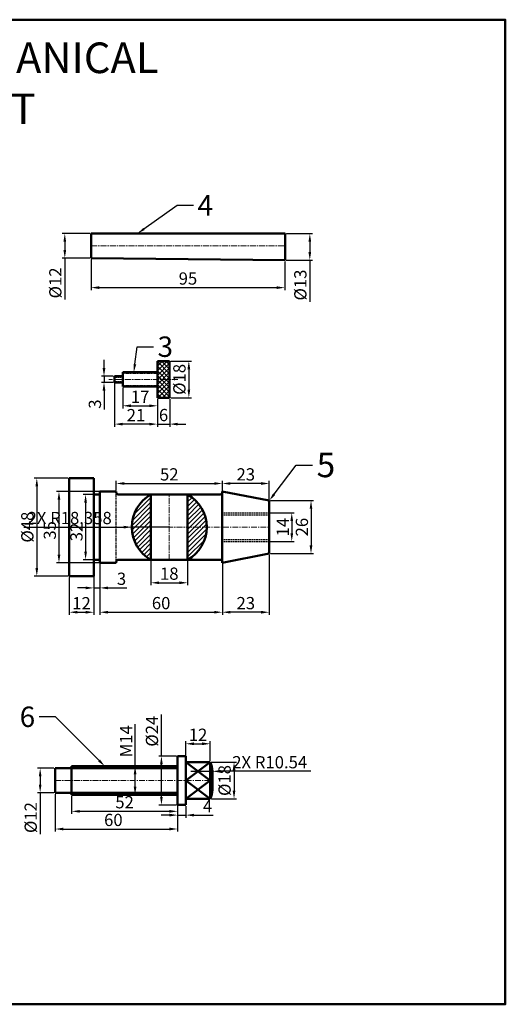
# Model space of a CAD drawing. Units: millimetres. Extents: x 197 to 841, y -182 to 351.
# Tile 3 of 3: x 603 to 841, y -132 to 351. Entities that reach past the tile are written whole.
import ezdxf
from ezdxf import colors
from ezdxf.entities.mleader import LeaderData, LeaderLine
from ezdxf.math import Vec2, Vec3

# ---------------------------------------------------------------- set-up
doc = ezdxf.new("R2010")
doc.units = ezdxf.units.MM
doc.header["$LTSCALE"] = 0.3
doc.linetypes.add('CENTER', pattern=[50.8, 31.75, -6.35, 6.35, -6.35])
doc.linetypes.add('HIDDEN', pattern=[9.525, 6.35, -3.175])
for name, color, linetype, lineweight in [('M-CNTR', 1, 'CENTER', 18), ('M-DIMS', 2, 'Continuous', 25), ('M-HATC', 8, 'Continuous', 18), ('M-HIDN', 6, 'HIDDEN', 25), ('M-OUTL', 7, 'Continuous', 50), ('M-TEXT', 3, 'Continuous', 25), ('M-TTLB', 7, 'Continuous', 50)]:
    doc.layers.add(name, color=color, linetype=linetype, lineweight=lineweight)
doc.styles.get("Standard").update_dxf_attribs({"font": 'arial.ttf'})
doc.dimstyles.new('ISO-25', dxfattribs={"dimtxt": 6, "dimasz": 4, "dimexe": 1.25, "dimexo": 0.625, "dimtad": 1, "dimdec": 0, "dimtxsty": 'Standard', "dimcen": 2.5, "dimadec": 0, "dimazin": 0, "dimtfac": 1, "dimtdec": 0, "dimtmove": 0, "dimatfit": 3, "dimfxl": 1, "dimarcsym": 0})

# ---------------------------------------------------------------- blocks, each defined once
blk = doc.blocks.new('*D37')
at = {"layer": 'Defpoints', "color": 0, "ltscale": 0.3, "transparency": 16777216}
for p in [(733.03, 245.93), (732.9, 232.93), (745.12, 232.93)]:
    blk.add_point(p, dxfattribs=at)
at = {"layer": 'M-DIMS', "color": 0, "lineweight": -2, "ltscale": 0.3, "transparency": 16777216}
for p, q in [((733.66, 245.93), (746.37, 245.93)), ((745.12, 241.93), (745.12, 236.93)), ((733.52, 232.93), (746.37, 232.93)), ((745.12, 232.93), (745.12, 212.55))]:
    blk.add_line(p, q, dxfattribs=at)
at = {"layer": 'M-DIMS', "color": 0, "ltscale": 0.3, "transparency": 16777216}
for points in [[(744.45, 241.93), (745.79, 241.93), (745.12, 245.93)], [(744.45, 236.93), (745.79, 236.93), (745.12, 232.93)]]:
    blk.add_solid(points, dxfattribs=at)
at = {"layer": 'M-DIMS', "color": 0, "ltscale": 0.3, "transparency": 16777216, "insert": (741.26, 220.74), "char_height": 6, "attachment_point": 5, "rotation": 90}
blk.add_mtext('%%C13', dxfattribs=at)
blk = doc.blocks.new('*D38')
at = {"layer": 'Defpoints', "color": 0, "ltscale": 0.3, "transparency": 16777216}
for p in [(638.03, 245.93), (625.05, 233.93), (637.91, 233.93)]:
    blk.add_point(p, dxfattribs=at)
at = {"layer": 'M-DIMS', "color": 0, "lineweight": -2, "ltscale": 0.3, "transparency": 16777216}
for p, q in [((637.41, 245.93), (623.8, 245.93)), ((625.05, 241.93), (625.05, 237.93)), ((637.28, 233.93), (623.8, 233.93)), ((625.05, 233.93), (625.05, 213.62))]:
    blk.add_line(p, q, dxfattribs=at)
at = {"layer": 'M-DIMS', "color": 0, "ltscale": 0.3, "transparency": 16777216}
for points in [[(624.38, 241.93), (625.71, 241.93), (625.05, 245.93)], [(624.38, 237.93), (625.71, 237.93), (625.05, 233.93)]]:
    blk.add_solid(points, dxfattribs=at)
at = {"layer": 'M-DIMS', "color": 0, "ltscale": 0.3, "transparency": 16777216, "insert": (621.19, 221.77), "char_height": 6, "attachment_point": 5, "rotation": 90}
blk.add_mtext('%%C12', dxfattribs=at)
blk = doc.blocks.new('*D39')
at = {"layer": 'Defpoints', "color": 0, "ltscale": 0.3, "transparency": 16777216}
for p in [(637.91, 233.93), (732.9, 232.93), (732.9, 219.47)]:
    blk.add_point(p, dxfattribs=at)
at = {"layer": 'M-DIMS', "color": 0, "lineweight": -2, "ltscale": 0.3, "transparency": 16777216}
for p, q in [((637.91, 233.3), (637.91, 218.22)), ((732.9, 232.3), (732.9, 218.22)), ((641.91, 219.47), (728.9, 219.47))]:
    blk.add_line(p, q, dxfattribs=at)
at = {"layer": 'M-DIMS', "color": 0, "ltscale": 0.3, "transparency": 16777216}
for points in [[(641.91, 220.14), (641.91, 218.81), (637.91, 219.47)], [(728.9, 220.14), (728.9, 218.81), (732.9, 219.47)]]:
    blk.add_solid(points, dxfattribs=at)
at = {"layer": 'M-DIMS', "color": 0, "ltscale": 0.3, "transparency": 16777216, "insert": (685.4, 223.16), "char_height": 6, "attachment_point": 5}
blk.add_mtext('95', dxfattribs=at)
blk = doc.blocks.new('*D40')
at = {"layer": 'Defpoints', "color": 0, "ltscale": 0.3, "transparency": 16777216}
for p in [(676.44, 183.51), (676.44, 165.51), (685.84, 165.51)]:
    blk.add_point(p, dxfattribs=at)
at = {"layer": 'M-DIMS', "color": 0, "lineweight": -2, "ltscale": 0.3, "transparency": 16777216}
for p, q in [((677.06, 183.51), (687.09, 183.51)), ((685.84, 179.51), (685.84, 169.51)), ((677.06, 165.51), (687.09, 165.51))]:
    blk.add_line(p, q, dxfattribs=at)
at = {"layer": 'M-DIMS', "color": 0, "ltscale": 0.3, "transparency": 16777216}
for points in [[(685.17, 179.51), (686.51, 179.51), (685.84, 183.51)], [(685.17, 169.51), (686.51, 169.51), (685.84, 165.51)]]:
    blk.add_solid(points, dxfattribs=at)
at = {"layer": 'M-DIMS', "color": 0, "ltscale": 0.3, "transparency": 16777216, "insert": (681.98, 174.51), "char_height": 6, "attachment_point": 5, "rotation": 90}
blk.add_mtext('%%C18', dxfattribs=at)
blk = doc.blocks.new('*D41')
at = {"layer": 'Defpoints', "color": 0, "ltscale": 0.3, "transparency": 16777216}
for p in [(653.44, 171.01), (670.44, 165.51), (670.44, 161.57)]:
    blk.add_point(p, dxfattribs=at)
at = {"layer": 'M-DIMS', "color": 0, "lineweight": -2, "ltscale": 0.3, "transparency": 16777216}
for p, q in [((653.44, 170.38), (653.44, 160.32)), ((670.44, 164.88), (670.44, 160.32)), ((657.44, 161.57), (666.44, 161.57))]:
    blk.add_line(p, q, dxfattribs=at)
at = {"layer": 'M-DIMS', "color": 0, "ltscale": 0.3, "transparency": 16777216}
for points in [[(657.44, 162.24), (657.44, 160.9), (653.44, 161.57)], [(666.44, 162.24), (666.44, 160.9), (670.44, 161.57)]]:
    blk.add_solid(points, dxfattribs=at)
at = {"layer": 'M-DIMS', "color": 0, "ltscale": 0.3, "transparency": 16777216, "insert": (661.94, 165.21), "char_height": 6, "attachment_point": 5}
blk.add_mtext('17', dxfattribs=at)
blk = doc.blocks.new('*D42')
at = {"layer": 'Defpoints', "color": 0, "ltscale": 0.3, "transparency": 16777216}
for p in [(670.44, 165.51), (676.44, 165.51), (676.44, 152.59)]:
    blk.add_point(p, dxfattribs=at)
at = {"layer": 'M-DIMS', "color": 0, "lineweight": -2, "ltscale": 0.3, "transparency": 16777216}
for p, q in [((670.44, 164.88), (670.44, 151.34)), ((676.44, 164.88), (676.44, 151.34)), ((666.44, 152.59), (662.44, 152.59)), ((670.44, 152.59), (676.44, 152.59)), ((680.44, 152.59), (684.44, 152.59))]:
    blk.add_line(p, q, dxfattribs=at)
at = {"layer": 'M-DIMS', "color": 0, "ltscale": 0.3, "transparency": 16777216}
for points in [[(666.44, 153.25), (666.44, 151.92), (670.44, 152.59)], [(680.44, 153.25), (680.44, 151.92), (676.44, 152.59)]]:
    blk.add_solid(points, dxfattribs=at)
at = {"layer": 'M-DIMS', "color": 0, "ltscale": 0.3, "transparency": 16777216, "insert": (673.44, 156.27), "char_height": 6, "attachment_point": 5}
blk.add_mtext('6', dxfattribs=at)
blk = doc.blocks.new('*D43')
at = {"layer": 'Defpoints', "color": 0, "ltscale": 0.3, "transparency": 16777216}
for p in [(649.44, 173.51), (670.44, 155.94), (649.44, 152.59)]:
    blk.add_point(p, dxfattribs=at)
at = {"layer": 'M-DIMS', "color": 0, "lineweight": -2, "ltscale": 0.3, "transparency": 16777216}
for p, q in [((649.44, 172.88), (649.44, 151.34)), ((670.44, 155.31), (670.44, 151.34)), ((666.44, 152.59), (653.44, 152.59))]:
    blk.add_line(p, q, dxfattribs=at)
at = {"layer": 'M-DIMS', "color": 0, "ltscale": 0.3, "transparency": 16777216}
for points in [[(653.44, 153.25), (653.44, 151.92), (649.44, 152.59)], [(666.44, 153.25), (666.44, 151.92), (670.44, 152.59)]]:
    blk.add_solid(points, dxfattribs=at)
at = {"layer": 'M-DIMS', "color": 0, "ltscale": 0.3, "transparency": 16777216, "insert": (659.94, 156.22), "char_height": 6, "attachment_point": 5}
blk.add_mtext('21', dxfattribs=at)
blk = doc.blocks.new('*D44')
at = {"layer": 'Defpoints', "color": 0, "ltscale": 0.3, "transparency": 16777216}
for p in [(649.44, 176.01), (644.26, 173.01), (649.44, 173.01)]:
    blk.add_point(p, dxfattribs=at)
at = {"layer": 'M-DIMS', "color": 0, "lineweight": -2, "ltscale": 0.3, "transparency": 16777216}
for p, q in [((644.26, 180.01), (644.26, 184.01)), ((648.81, 176.01), (643.01, 176.01)), ((644.26, 176.01), (644.26, 173.01)), ((648.81, 173.01), (643.01, 173.01)), ((644.26, 169.01), (644.26, 159.83))]:
    blk.add_line(p, q, dxfattribs=at)
at = {"layer": 'M-DIMS', "color": 0, "ltscale": 0.3, "transparency": 16777216}
for points in [[(643.59, 180.01), (644.93, 180.01), (644.26, 176.01)], [(643.59, 169.01), (644.93, 169.01), (644.26, 173.01)]]:
    blk.add_solid(points, dxfattribs=at)
at = {"layer": 'M-DIMS', "color": 0, "ltscale": 0.3, "transparency": 16777216, "insert": (640.57, 162.42), "char_height": 6, "attachment_point": 5, "rotation": 90}
blk.add_mtext('3', dxfattribs=at)
blk = doc.blocks.new('*D45')
at = {"layer": 'Defpoints', "color": 0, "ltscale": 0.3, "transparency": 16777216}
for p in [(725.25, 109.12), (725.25, 95.12), (736.27, 95.12)]:
    blk.add_point(p, dxfattribs=at)
at = {"layer": 'M-DIMS', "color": 0, "lineweight": -2, "ltscale": 0.3, "transparency": 16777216}
for p, q in [((725.87, 109.12), (737.52, 109.12)), ((736.27, 105.12), (736.27, 99.12)), ((725.87, 95.12), (737.52, 95.12))]:
    blk.add_line(p, q, dxfattribs=at)
at = {"layer": 'M-DIMS', "color": 0, "ltscale": 0.3, "transparency": 16777216}
for points in [[(735.61, 105.12), (736.94, 105.12), (736.27, 109.12)], [(735.61, 99.12), (736.94, 99.12), (736.27, 95.12)]]:
    blk.add_solid(points, dxfattribs=at)
at = {"layer": 'M-DIMS', "color": 0, "ltscale": 0.3, "transparency": 16777216, "insert": (732.64, 102.12), "char_height": 6, "attachment_point": 5, "rotation": 90}
blk.add_mtext('14', dxfattribs=at)
blk = doc.blocks.new('*D46')
at = {"layer": 'Defpoints', "color": 0, "ltscale": 0.3, "transparency": 16777216}
for p in [(725.25, 115.12), (725.25, 89.12), (745.71, 89.12)]:
    blk.add_point(p, dxfattribs=at)
at = {"layer": 'M-DIMS', "color": 0, "lineweight": -2, "ltscale": 0.3, "transparency": 16777216}
for p, q in [((725.87, 115.12), (746.96, 115.12)), ((745.71, 111.12), (745.71, 93.12)), ((725.87, 89.12), (746.96, 89.12))]:
    blk.add_line(p, q, dxfattribs=at)
at = {"layer": 'M-DIMS', "color": 0, "ltscale": 0.3, "transparency": 16777216}
for points in [[(745.04, 111.12), (746.37, 111.12), (745.71, 115.12)], [(745.04, 93.12), (746.37, 93.12), (745.71, 89.12)]]:
    blk.add_solid(points, dxfattribs=at)
at = {"layer": 'M-DIMS', "color": 0, "ltscale": 0.3, "transparency": 16777216, "insert": (742.02, 102.12), "char_height": 6, "attachment_point": 5, "rotation": 90}
blk.add_mtext('26', dxfattribs=at)
blk = doc.blocks.new('*D47')
at = {"layer": 'Defpoints', "color": 0, "ltscale": 0.3, "transparency": 16777216}
for p in [(627.25, 78.12), (639.25, 78.12), (639.25, 60.41)]:
    blk.add_point(p, dxfattribs=at)
at = {"layer": 'M-DIMS', "color": 0, "lineweight": -2, "ltscale": 0.3, "transparency": 16777216}
for p, q in [((627.25, 77.49), (627.25, 59.16)), ((639.25, 77.49), (639.25, 59.16)), ((631.25, 60.41), (635.25, 60.41))]:
    blk.add_line(p, q, dxfattribs=at)
at = {"layer": 'M-DIMS', "color": 0, "ltscale": 0.3, "transparency": 16777216}
for points in [[(631.25, 61.08), (631.25, 59.75), (627.25, 60.41)], [(635.25, 61.08), (635.25, 59.75), (639.25, 60.41)]]:
    blk.add_solid(points, dxfattribs=at)
at = {"layer": 'M-DIMS', "color": 0, "ltscale": 0.3, "transparency": 16777216, "insert": (633.25, 64.05), "char_height": 6, "attachment_point": 5}
blk.add_mtext('12', dxfattribs=at)
blk = doc.blocks.new('*D48')
at = {"layer": 'Defpoints', "color": 0, "ltscale": 0.3, "transparency": 16777216}
for p in [(639.25, 86.12), (642.25, 86.12), (642.25, 72.34)]:
    blk.add_point(p, dxfattribs=at)
at = {"layer": 'M-DIMS', "color": 0, "lineweight": -2, "ltscale": 0.3, "transparency": 16777216}
for p, q in [((639.25, 85.49), (639.25, 71.09)), ((642.25, 85.49), (642.25, 71.09)), ((635.25, 72.34), (631.25, 72.34)), ((639.25, 72.34), (642.25, 72.34)), ((646.25, 72.34), (655.42, 72.34))]:
    blk.add_line(p, q, dxfattribs=at)
at = {"layer": 'M-DIMS', "color": 0, "ltscale": 0.3, "transparency": 16777216}
for points in [[(635.25, 73), (635.25, 71.67), (639.25, 72.34)], [(646.25, 73), (646.25, 71.67), (642.25, 72.34)]]:
    blk.add_solid(points, dxfattribs=at)
at = {"layer": 'M-DIMS', "color": 0, "ltscale": 0.3, "transparency": 16777216, "insert": (652.84, 76.03), "char_height": 6, "attachment_point": 5}
blk.add_mtext('3', dxfattribs=at)
blk = doc.blocks.new('*D49')
at = {"layer": 'Defpoints', "color": 0, "ltscale": 0.3, "transparency": 16777216}
for p in [(642.25, 90.66), (702.25, 90.66), (702.25, 60.41)]:
    blk.add_point(p, dxfattribs=at)
at = {"layer": 'M-DIMS', "color": 0, "lineweight": -2, "ltscale": 0.3, "transparency": 16777216}
for p, q in [((642.25, 90.03), (642.25, 59.16)), ((702.25, 90.03), (702.25, 59.16)), ((646.25, 60.41), (698.25, 60.41))]:
    blk.add_line(p, q, dxfattribs=at)
at = {"layer": 'M-DIMS', "color": 0, "ltscale": 0.3, "transparency": 16777216}
for points in [[(646.25, 61.08), (646.25, 59.75), (642.25, 60.41)], [(698.25, 61.08), (698.25, 59.75), (702.25, 60.41)]]:
    blk.add_solid(points, dxfattribs=at)
at = {"layer": 'M-DIMS', "color": 0, "ltscale": 0.3, "transparency": 16777216, "insert": (672.25, 64.1), "char_height": 6, "attachment_point": 5}
blk.add_mtext('60', dxfattribs=at)
blk = doc.blocks.new('*D50')
at = {"layer": 'Defpoints', "color": 0, "ltscale": 0.3, "transparency": 16777216}
for p in [(725.25, 89.12), (702.25, 74.6), (702.25, 60.41)]:
    blk.add_point(p, dxfattribs=at)
at = {"layer": 'M-DIMS', "color": 0, "lineweight": -2, "ltscale": 0.3, "transparency": 16777216}
for p, q in [((725.25, 88.49), (725.25, 59.16)), ((702.25, 73.97), (702.25, 59.16)), ((721.25, 60.41), (706.25, 60.41))]:
    blk.add_line(p, q, dxfattribs=at)
at = {"layer": 'M-DIMS', "color": 0, "ltscale": 0.3, "transparency": 16777216}
for points in [[(706.25, 61.08), (706.25, 59.75), (702.25, 60.41)], [(721.25, 61.08), (721.25, 59.75), (725.25, 60.41)]]:
    blk.add_solid(points, dxfattribs=at)
at = {"layer": 'M-DIMS', "color": 0, "ltscale": 0.3, "transparency": 16777216, "insert": (713.75, 64.1), "char_height": 6, "attachment_point": 5}
blk.add_mtext('23', dxfattribs=at)
blk = doc.blocks.new('*D51')
at = {"layer": 'Defpoints', "color": 0, "ltscale": 0.3, "transparency": 16777216}
for p in [(650.25, 119.62), (622.19, 84.62), (650.25, 84.62)]:
    blk.add_point(p, dxfattribs=at)
at = {"layer": 'M-DIMS', "color": 0, "lineweight": -2, "ltscale": 0.3, "transparency": 16777216}
for p, q in [((649.62, 119.62), (620.94, 119.62)), ((622.19, 115.62), (622.19, 88.62)), ((649.62, 84.62), (620.94, 84.62))]:
    blk.add_line(p, q, dxfattribs=at)
at = {"layer": 'M-DIMS', "color": 0, "ltscale": 0.3, "transparency": 16777216}
for points in [[(621.52, 115.62), (622.85, 115.62), (622.19, 119.62)], [(621.52, 88.62), (622.85, 88.62), (622.19, 84.62)]]:
    blk.add_solid(points, dxfattribs=at)
at = {"layer": 'M-DIMS', "color": 0, "ltscale": 0.3, "transparency": 16777216, "insert": (618.49, 100.53), "char_height": 6, "attachment_point": 5, "rotation": 90}
blk.add_mtext('35', dxfattribs=at)
blk = doc.blocks.new('*D52')
at = {"layer": 'Defpoints', "color": 0, "ltscale": 0.3, "transparency": 16777216}
for p in [(702.25, 123.5), (650.25, 119.37), (702.25, 119.62)]:
    blk.add_point(p, dxfattribs=at)
at = {"layer": 'M-DIMS', "color": 0, "lineweight": -2, "ltscale": 0.3, "transparency": 16777216}
for p, q in [((650.25, 119.99), (650.25, 124.75)), ((654.25, 123.5), (698.25, 123.5)), ((702.25, 120.24), (702.25, 124.75))]:
    blk.add_line(p, q, dxfattribs=at)
at = {"layer": 'M-DIMS', "color": 0, "ltscale": 0.3, "transparency": 16777216}
for points in [[(654.25, 124.17), (654.25, 122.83), (650.25, 123.5)], [(698.25, 124.17), (698.25, 122.83), (702.25, 123.5)]]:
    blk.add_solid(points, dxfattribs=at)
at = {"layer": 'M-DIMS', "color": 0, "ltscale": 0.3, "transparency": 16777216, "insert": (676.25, 127.19), "char_height": 6, "attachment_point": 5}
blk.add_mtext('52', dxfattribs=at)
blk = doc.blocks.new('*D53')
at = {"layer": 'Defpoints', "color": 0, "ltscale": 0.3, "transparency": 16777216}
for p in [(702.25, 123.5), (702.25, 115.12), (725.25, 115.12)]:
    blk.add_point(p, dxfattribs=at)
at = {"layer": 'M-DIMS', "color": 0, "lineweight": -2, "ltscale": 0.3, "transparency": 16777216}
for p, q in [((702.25, 115.74), (702.25, 124.75)), ((721.25, 123.5), (706.25, 123.5)), ((725.25, 115.74), (725.25, 124.75))]:
    blk.add_line(p, q, dxfattribs=at)
at = {"layer": 'M-DIMS', "color": 0, "ltscale": 0.3, "transparency": 16777216}
for points in [[(706.25, 124.17), (706.25, 122.83), (702.25, 123.5)], [(721.25, 124.17), (721.25, 122.83), (725.25, 123.5)]]:
    blk.add_solid(points, dxfattribs=at)
at = {"layer": 'M-DIMS', "color": 0, "ltscale": 0.3, "transparency": 16777216, "insert": (713.75, 127.19), "char_height": 6, "attachment_point": 5}
blk.add_mtext('23', dxfattribs=at)
blk = doc.blocks.new('*D54')
at = {"layer": 'Defpoints', "color": 0, "ltscale": 0.3, "transparency": 16777216}
for p in [(639.25, 118.12), (635.24, 86.12), (639.25, 86.12)]:
    blk.add_point(p, dxfattribs=at)
at = {"layer": 'M-DIMS', "color": 0, "lineweight": -2, "ltscale": 0.3, "transparency": 16777216}
for p, q in [((638.62, 118.12), (633.99, 118.12)), ((635.24, 114.12), (635.24, 90.12)), ((638.62, 86.12), (633.99, 86.12))]:
    blk.add_line(p, q, dxfattribs=at)
at = {"layer": 'M-DIMS', "color": 0, "ltscale": 0.3, "transparency": 16777216}
for points in [[(634.58, 114.12), (635.91, 114.12), (635.24, 118.12)], [(634.58, 90.12), (635.91, 90.12), (635.24, 86.12)]]:
    blk.add_solid(points, dxfattribs=at)
at = {"layer": 'M-DIMS', "color": 0, "ltscale": 0.3, "transparency": 16777216, "insert": (631.55, 99.72), "char_height": 6, "attachment_point": 5, "rotation": 90}
blk.add_mtext('32', dxfattribs=at)
blk = doc.blocks.new('*D55')
at = {"layer": 'Defpoints', "color": 0, "ltscale": 0.3, "transparency": 16777216}
for p in [(627.25, 126.12), (611.32, 78.12), (627.25, 78.12)]:
    blk.add_point(p, dxfattribs=at)
at = {"layer": 'M-DIMS', "color": 0, "lineweight": -2, "ltscale": 0.3, "transparency": 16777216}
for p, q in [((626.62, 126.12), (610.07, 126.12)), ((611.32, 122.12), (611.32, 82.12)), ((626.62, 78.12), (610.07, 78.12))]:
    blk.add_line(p, q, dxfattribs=at)
at = {"layer": 'M-DIMS', "color": 0, "ltscale": 0.3, "transparency": 16777216}
for points in [[(610.66, 122.12), (611.99, 122.12), (611.32, 126.12)], [(610.66, 82.12), (611.99, 82.12), (611.32, 78.12)]]:
    blk.add_solid(points, dxfattribs=at)
at = {"layer": 'M-DIMS', "color": 0, "ltscale": 0.3, "transparency": 16777216, "insert": (607.47, 102.12), "char_height": 6, "attachment_point": 5, "rotation": 90}
blk.add_mtext('%%C48', dxfattribs=at)
blk = doc.blocks.new('*D56')
at = {"layer": 'Defpoints', "color": 0, "ltscale": 0.3, "transparency": 16777216}
for p in [(667.25, 86.12), (685.25, 86.12), (685.25, 74.85)]:
    blk.add_point(p, dxfattribs=at)
at = {"layer": 'M-DIMS', "color": 0, "lineweight": -2, "ltscale": 0.3, "transparency": 16777216}
for p, q in [((667.25, 85.49), (667.25, 73.6)), ((685.25, 85.49), (685.25, 73.6)), ((671.25, 74.85), (681.25, 74.85))]:
    blk.add_line(p, q, dxfattribs=at)
at = {"layer": 'M-DIMS', "color": 0, "ltscale": 0.3, "transparency": 16777216}
for points in [[(671.25, 75.52), (671.25, 74.19), (667.25, 74.85)], [(681.25, 75.52), (681.25, 74.19), (685.25, 74.85)]]:
    blk.add_solid(points, dxfattribs=at)
at = {"layer": 'M-DIMS', "color": 0, "ltscale": 0.3, "transparency": 16777216, "insert": (676.25, 78.54), "char_height": 6, "attachment_point": 5}
blk.add_mtext('18', dxfattribs=at)
blk = doc.blocks.new('*D57')
at = {"layer": 'Defpoints', "color": 0, "ltscale": 0.3, "transparency": 16777216}
for p in [(696.35, -13.04), (696.35, -31.04), (707.98, -31.04)]:
    blk.add_point(p, dxfattribs=at)
at = {"layer": 'M-DIMS', "color": 0, "lineweight": -2, "ltscale": 0.3, "transparency": 16777216}
for p, q in [((696.98, -13.04), (709.23, -13.04)), ((707.98, -17.04), (707.98, -27.04)), ((696.98, -31.04), (709.23, -31.04))]:
    blk.add_line(p, q, dxfattribs=at)
at = {"layer": 'M-DIMS', "color": 0, "ltscale": 0.3, "transparency": 16777216}
for points in [[(707.32, -17.04), (708.65, -17.04), (707.98, -13.04)], [(707.32, -27.04), (708.65, -27.04), (707.98, -31.04)]]:
    blk.add_solid(points, dxfattribs=at)
at = {"layer": 'M-DIMS', "color": 0, "ltscale": 0.3, "transparency": 16777216, "insert": (704.13, -22.04), "char_height": 6, "attachment_point": 5, "rotation": 90}
blk.add_mtext('%%C18', dxfattribs=at)
blk = doc.blocks.new('*D58')
at = {"layer": 'Defpoints', "color": 0, "ltscale": 0.3, "transparency": 16777216}
for p in [(680.35, -10.04), (672.4, -34.04), (680.35, -34.04)]:
    blk.add_point(p, dxfattribs=at)
at = {"layer": 'M-DIMS', "color": 0, "lineweight": -2, "ltscale": 0.3, "transparency": 16777216}
for p, q in [((672.4, -10.04), (672.4, 10.31)), ((679.73, -10.04), (671.15, -10.04)), ((672.4, -30.04), (672.4, -14.04)), ((679.73, -34.04), (671.15, -34.04))]:
    blk.add_line(p, q, dxfattribs=at)
at = {"layer": 'M-DIMS', "color": 0, "ltscale": 0.3, "transparency": 16777216}
for points in [[(671.73, -14.04), (673.06, -14.04), (672.4, -10.04)], [(671.73, -30.04), (673.06, -30.04), (672.4, -34.04)]]:
    blk.add_solid(points, dxfattribs=at)
at = {"layer": 'M-DIMS', "color": 0, "ltscale": 0.3, "transparency": 16777216, "insert": (668.54, 2.13), "char_height": 6, "width": 8.9781, "attachment_point": 5, "rotation": 90}
blk.add_mtext('%%C24', dxfattribs=at)
blk = doc.blocks.new('*D59')
at = {"layer": 'Defpoints', "color": 0, "ltscale": 0.3, "transparency": 16777216}
for p in [(658, -15.04), (658, -29.04), (659.5, -29.04)]:
    blk.add_point(p, dxfattribs=at)
at = {"layer": 'M-DIMS', "color": 0, "lineweight": -2, "ltscale": 0.3, "transparency": 16777216}
for p, q in [((659.5, -15.04), (659.5, 5.49)), ((658.62, -15.04), (660.75, -15.04)), ((659.5, -25.04), (659.5, -19.04)), ((658.62, -29.04), (660.75, -29.04))]:
    blk.add_line(p, q, dxfattribs=at)
at = {"layer": 'M-DIMS', "color": 0, "ltscale": 0.3, "transparency": 16777216}
for points in [[(658.83, -19.04), (660.17, -19.04), (659.5, -15.04)], [(658.83, -25.04), (660.17, -25.04), (659.5, -29.04)]]:
    blk.add_solid(points, dxfattribs=at)
at = {"layer": 'M-DIMS', "color": 0, "ltscale": 0.3, "transparency": 16777216, "insert": (655.86, -2.78), "char_height": 6, "attachment_point": 5, "rotation": 90}
blk.add_mtext('M14', dxfattribs=at)
blk = doc.blocks.new('*D60')
at = {"layer": 'Defpoints', "color": 0, "ltscale": 0.3, "transparency": 16777216}
for p in [(620.35, -28.04), (680.35, -34.04), (680.35, -45.81)]:
    blk.add_point(p, dxfattribs=at)
at = {"layer": 'M-DIMS', "color": 0, "lineweight": -2, "ltscale": 0.3, "transparency": 16777216}
for p, q in [((620.35, -28.66), (620.35, -47.06)), ((680.35, -34.66), (680.35, -47.06)), ((624.35, -45.81), (676.35, -45.81))]:
    blk.add_line(p, q, dxfattribs=at)
at = {"layer": 'M-DIMS', "color": 0, "ltscale": 0.3, "transparency": 16777216}
for points in [[(624.35, -45.14), (624.35, -46.47), (620.35, -45.81)], [(676.35, -45.14), (676.35, -46.47), (680.35, -45.81)]]:
    blk.add_solid(points, dxfattribs=at)
at = {"layer": 'M-DIMS', "color": 0, "ltscale": 0.3, "transparency": 16777216, "insert": (648.85, -42.12), "char_height": 6, "attachment_point": 5}
blk.add_mtext('60', dxfattribs=at)
blk = doc.blocks.new('*D61')
at = {"layer": 'Defpoints', "color": 0, "ltscale": 0.3, "transparency": 16777216}
for p in [(680.35, -34.04), (684.35, -34.04), (684.35, -39)]:
    blk.add_point(p, dxfattribs=at)
at = {"layer": 'M-DIMS', "color": 0, "lineweight": -2, "ltscale": 0.3, "transparency": 16777216}
for p, q in [((680.35, -34.66), (680.35, -40.25)), ((684.35, -34.66), (684.35, -40.25)), ((676.35, -39), (672.35, -39)), ((680.35, -39), (684.35, -39)), ((688.35, -39), (697.75, -39))]:
    blk.add_line(p, q, dxfattribs=at)
at = {"layer": 'M-DIMS', "color": 0, "ltscale": 0.3, "transparency": 16777216}
for points in [[(676.35, -38.33), (676.35, -39.66), (680.35, -39)], [(688.35, -38.33), (688.35, -39.66), (684.35, -39)]]:
    blk.add_solid(points, dxfattribs=at)
at = {"layer": 'M-DIMS', "color": 0, "ltscale": 0.3, "transparency": 16777216, "insert": (695.05, -35.37), "char_height": 6, "attachment_point": 5}
blk.add_mtext('4', dxfattribs=at)
blk = doc.blocks.new('*D62')
at = {"layer": 'Defpoints', "color": 0, "ltscale": 0.3, "transparency": 16777216}
for p in [(620.35, -16.04), (612.98, -28.04), (620.35, -28.04)]:
    blk.add_point(p, dxfattribs=at)
at = {"layer": 'M-DIMS', "color": 0, "lineweight": -2, "ltscale": 0.3, "transparency": 16777216}
for p, q in [((619.73, -16.04), (611.73, -16.04)), ((612.98, -20.04), (612.98, -24.04)), ((619.73, -28.04), (611.73, -28.04)), ((612.98, -28.04), (612.98, -48.35))]:
    blk.add_line(p, q, dxfattribs=at)
at = {"layer": 'M-DIMS', "color": 0, "ltscale": 0.3, "transparency": 16777216}
for points in [[(612.31, -20.04), (613.64, -20.04), (612.98, -16.04)], [(612.31, -24.04), (613.64, -24.04), (612.98, -28.04)]]:
    blk.add_solid(points, dxfattribs=at)
at = {"layer": 'M-DIMS', "color": 0, "ltscale": 0.3, "transparency": 16777216, "insert": (609.12, -40.2), "char_height": 6, "attachment_point": 5, "rotation": 90}
blk.add_mtext('%%C12', dxfattribs=at)
blk = doc.blocks.new('*D63')
at = {"layer": 'Defpoints', "color": 0, "ltscale": 0.3, "transparency": 16777216}
for p in [(628.35, -29.04), (680.35, -31.97), (680.35, -37.14)]:
    blk.add_point(p, dxfattribs=at)
at = {"layer": 'M-DIMS', "color": 0, "lineweight": -2, "ltscale": 0.3, "transparency": 16777216}
for p, q in [((628.35, -29.66), (628.35, -38.39)), ((680.35, -32.6), (680.35, -38.39)), ((632.35, -37.14), (676.35, -37.14))]:
    blk.add_line(p, q, dxfattribs=at)
at = {"layer": 'M-DIMS', "color": 0, "ltscale": 0.3, "transparency": 16777216}
for points in [[(632.35, -36.48), (632.35, -37.81), (628.35, -37.14)], [(676.35, -36.48), (676.35, -37.81), (680.35, -37.14)]]:
    blk.add_solid(points, dxfattribs=at)
at = {"layer": 'M-DIMS', "color": 0, "ltscale": 0.3, "transparency": 16777216, "insert": (654.35, -33.46), "char_height": 6, "attachment_point": 5}
blk.add_mtext('52', dxfattribs=at)
blk = doc.blocks.new('*D66')
at = {"layer": 'Defpoints', "color": 0, "ltscale": 0.3, "transparency": 16777216}
for p in [(696.35, -4.04), (684.35, -13.04), (696.35, -13.04)]:
    blk.add_point(p, dxfattribs=at)
at = {"layer": 'M-DIMS', "color": 0, "lineweight": -2, "ltscale": 0.3, "transparency": 16777216}
for p, q in [((684.35, -12.41), (684.35, -2.79)), ((688.35, -4.04), (692.35, -4.04)), ((696.35, -12.41), (696.35, -2.79))]:
    blk.add_line(p, q, dxfattribs=at)
at = {"layer": 'M-DIMS', "color": 0, "ltscale": 0.3, "transparency": 16777216}
for points in [[(688.35, -3.37), (688.35, -4.71), (684.35, -4.04)], [(692.35, -3.37), (692.35, -4.71), (696.35, -4.04)]]:
    blk.add_solid(points, dxfattribs=at)
at = {"layer": 'M-DIMS', "color": 0, "ltscale": 0.3, "transparency": 16777216, "insert": (690.35, -0.4), "char_height": 6, "attachment_point": 5}
blk.add_mtext('12', dxfattribs=at)
blk = doc.blocks.new('*D78')
at = {"layer": 'Defpoints', "color": 0, "ltscale": 0.3, "transparency": 16777216}
for p in [(657.89, 102.12), (676.25, 102.12)]:
    blk.add_point(p, dxfattribs=at)
at = {"layer": 'M-DIMS', "color": 0, "lineweight": -2, "ltscale": 0.3, "transparency": 16777216}
for p, q in [((604.98, 102.12), (653.89, 102.12)), ((676.25, 102.12), (657.89, 102.12))]:
    blk.add_line(p, q, dxfattribs=at)
at = {"layer": 'M-DIMS', "color": 0, "ltscale": 0.3, "transparency": 16777216}
blk.add_solid([(653.89, 102.78), (653.89, 101.45), (657.89, 102.12)], dxfattribs=at)
at = {"layer": 'M-DIMS', "color": 0, "ltscale": 0.3, "transparency": 16777216, "insert": (627.43, 105.81), "char_height": 6, "attachment_point": 5, "rotation": 359.9984}
blk.add_mtext('2X R18.358', dxfattribs=at)
blk = doc.blocks.new('*D79')
at = {"layer": 'Defpoints', "color": 0, "ltscale": 0.3, "transparency": 16777216}
for p in [(686.82, -17.54), (697.36, -17.54)]:
    blk.add_point(p, dxfattribs=at)
at = {"layer": 'M-DIMS', "color": 0, "lineweight": -2, "ltscale": 0.3, "transparency": 16777216}
for p, q in [((686.82, -17.54), (697.36, -17.54)), ((745.57, -17.54), (701.36, -17.54))]:
    blk.add_line(p, q, dxfattribs=at)
at = {"layer": 'M-DIMS', "color": 0, "ltscale": 0.3, "transparency": 16777216}
blk.add_solid([(701.36, -16.87), (701.36, -18.21), (697.36, -17.54)], dxfattribs=at)
at = {"layer": 'M-DIMS', "color": 0, "ltscale": 0.3, "transparency": 16777216, "insert": (725.46, -13.85), "char_height": 6, "attachment_point": 5, "rotation": 359.9986}
blk.add_mtext('2X R10.54', dxfattribs=at)

msp = doc.modelspace()

# ---------------------------------------------------------------- hatches: boundary and pattern name
at = {"layer": 'M-HATC', "ltscale": 0.3}
h = msp.add_hatch(dxfattribs=at)
h.set_pattern_fill('ANSI37', color=256, scale=0.5)
h.set_pattern_definition([(45, (-40.1366, 72.0882), (-1.122532, 1.122532), []), (135, (-40.1366, 72.0882), (-1.122532, -1.122532), [])])
h.paths.add_polyline_path([(676.4377, 174.5071), (670.4377, 174.5071), (670.4377, 165.5071), (676.4377, 165.5071)])
h.paths.add_polyline_path([(676.4377, 183.5071), (670.4377, 183.5071), (670.4377, 174.5071), (676.4377, 174.5071)])
h = msp.add_hatch(dxfattribs=at)
h.set_pattern_fill('ANSI31', color=256, scale=0.5)
h.set_pattern_definition([(45, (-62.6375, 35.6014), (-1.122532, 1.122532), [])])
h.paths.add_polyline_path([(667.2456, 118.1155, 0.27095498), (657.888, 102.1155), (667.2456, 102.1155)])
h.paths.add_polyline_path([(667.2456, 102.1155), (657.888, 102.1155, 0.27095498), (667.2456, 86.1155)])
h.paths.add_polyline_path([(685.2456, 118.1155), (685.2456, 102.1155), (694.6031, 102.1155, 0.27095498)])
h.paths.add_polyline_path([(694.6031, 102.1155), (685.2456, 102.1155), (685.2456, 86.1155, 0.27095498)])

# ---------------------------------------------------------------- linework, layer by layer
at = {"layer": 'M-CNTR', "ltscale": 0.3}
for p, q in [((638.0338, 239.9254), (732.9477, 239.9254)), ((680.42, 174.5071), (646.6095, 174.5071)), ((676.2456, 86.1155), (676.2456, 118.1155)), ((620.3558, 102.1155), (725.2456, 102.1155)), ((696.3504, -22.0397), (620.3504, -22.0397))]:
    msp.add_line(p, q, dxfattribs=at)
at = {"layer": 'M-HIDN', "ltscale": 0.3}
for p, q in [((653.4377, 175.5071), (649.4377, 175.5071)), ((653.4377, 177.5071), (670.4377, 177.5071)), ((649.4377, 173.5071), (653.4377, 173.5071)), ((653.4377, 171.5071), (670.4377, 171.5071)), ((650.2456, 85.1155), (650.2456, 119.6155)), ((702.2456, 109.1155), (725.2456, 109.1155)), ((702.2456, 108.1155), (725.2456, 108.1155)), ((702.2456, 96.1155), (725.2456, 96.1155)), ((702.2456, 95.1155), (725.2456, 95.1155))]:
    msp.add_line(p, q, dxfattribs=at)
at = {"layer": 'M-OUTL', "ltscale": 0.3}
for p, q in [((638.0338, 245.9254), (638.0338, 233.9254)), ((638.0338, 245.9254), (733.0338, 245.9254)), ((733.0338, 245.9254), (733.0338, 232.9254)), ((733.0338, 232.9254), (638.0338, 233.9254)), ((670.4377, 183.5071), (676.4377, 183.5071)), ((670.4377, 165.5071), (670.4377, 183.5071)), ((676.4377, 183.5071), (676.4377, 165.5071)), ((653.4377, 176.0071), (649.4377, 176.0071)), ((649.4377, 176.0071), (649.4377, 174.5071)), ((649.4377, 174.5071), (649.4377, 173.0071)), ((653.4377, 174.5071), (653.4377, 178.0071)), ((653.4377, 178.0071), (670.4377, 178.0071)), ((653.4377, 173.0071), (653.4377, 176.0071)), ((653.4377, 174.5071), (653.4377, 171.0071)), ((649.4377, 173.0071), (653.4377, 173.0071)), ((653.4377, 171.0071), (670.4377, 171.0071)), ((676.4377, 165.5071), (670.4377, 165.5071)), ((627.2456, 126.1155), (627.2456, 78.1155)), ((639.2456, 126.1155), (627.2456, 126.1155)), ((639.2456, 78.1155), (639.2456, 126.1155)), ((639.2456, 118.1155), (639.2456, 86.1155)), ((642.2456, 118.1155), (639.2456, 118.1155)), ((650.2456, 119.6155), (642.2456, 119.6155)), ((642.2456, 119.6155), (642.2456, 118.1155)), ((642.2456, 86.1155), (642.2456, 118.1155)), ((650.2456, 119.1155), (650.2456, 119.6155)), ((651.2456, 118.1155), (701.2456, 118.1155)), ((667.2456, 86.1155), (667.2456, 118.1155)), ((685.2456, 86.1155), (685.2456, 118.1155)), ((725.2456, 115.1155), (702.2456, 119.6155)), ((702.2456, 119.1155), (702.2456, 119.6155)), ((702.2456, 119.6155), (702.2456, 85.1155)), ((725.2456, 102.1155), (725.2456, 115.1155)), ((725.2456, 102.1155), (725.2456, 89.1155)), ((725.2456, 89.1155), (702.2456, 84.6155)), ((639.2456, 86.1155), (642.2456, 86.1155)), ((642.2456, 84.6155), (642.2456, 86.1155)), ((650.2456, 84.6155), (642.2456, 84.6155)), ((650.2456, 84.6155), (650.2456, 85.1155)), ((651.2456, 86.1155), (701.2456, 86.1155)), ((702.2456, 84.6155), (702.2456, 85.1155)), ((627.2456, 78.1155), (639.2456, 78.1155)), ((680.3504, -10.0397), (680.3504, -34.0397)), ((684.3504, -10.0397), (680.3504, -10.0397)), ((684.3504, -34.0397), (684.3504, -10.0397)), ((696.3504, -13.0397), (684.3504, -13.0397)), ((684.3504, -13.0397), (696.3504, -22.0397)), ((684.3504, -22.0397), (696.3504, -13.0397)), ((696.3504, -31.0397), (696.3504, -13.0397)), ((620.3504, -28.0397), (620.3504, -16.0397)), ((620.3504, -16.0397), (628.3504, -16.0397)), ((628.3504, -22.0397), (628.3504, -15.0397)), ((628.3504, -15.0397), (680.3504, -15.0397)), ((628.3504, -16.0397), (680.3504, -16.0397)), ((697.3504, -26.9743), (697.3504, -17.1051)), ((628.3504, -22.0397), (628.3504, -29.0397)), ((696.3504, -22.0397), (684.3504, -31.0397)), ((696.3504, -31.0397), (684.3504, -22.0397)), ((620.3504, -28.0397), (628.3504, -28.0397)), ((628.3504, -28.0397), (680.3504, -28.0397)), ((628.3504, -29.0397), (680.3504, -29.0397)), ((696.3504, -31.0397), (684.3504, -31.0397)), ((680.3504, -34.0397), (684.3504, -34.0397))]:
    msp.add_line(p, q, dxfattribs=at)
for centre, radius, start, end in [((651.2456, 119.1155), 1, 180, 270), ((676.2456, 102.1155), 18.3576, 119.357754, 240.642246), ((676.2456, 102.1155), 18.3576, 299.357754, 60.642246), ((701.2456, 119.1155), 1, 270, 0), ((651.2456, 85.1155), 1, 90, 180), ((701.2456, 85.1155), 1, 0, 90), ((686.8199, -17.5397), 10.5395, 334.724944, 25.275056), ((686.8199, -26.5397), 10.5395, 334.724944, 25.275056)]:
    msp.add_arc(centre, radius, start, end, dxfattribs=at)
at = {"layer": 'M-TTLB', "ltscale": 0.3}
msp.add_lwpolyline([(196.5121, 350.7597), (840.9228, 350.7597), (840.9228, -131.7005), (196.5121, -131.7005)], close=True, dxfattribs=at)

# ---------------------------------------------------------------- texts
at = {"layer": 'M-TEXT', "ltscale": 0.3, "insert": (410.4687, 339.5846), "char_height": 15, "attachment_point": 1}
msp.add_mtext_dynamic_manual_height_columns('\\pxqc;ASSEMBLED MECHANICAL COMPONENT', width=273.781942, gutter_width=12.5, heights=[0], dxfattribs=at)

# ---------------------------------------------------------------- dimensions: what is measured, and where the dimension line sits
at = {"layer": 'M-DIMS', "ltscale": 0.3}
for base, p1, p2, picture, middle in [((625.0451, 233.9267), (638.0338, 245.9254), (637.9075, 233.9267), '*D38', (621.1889, 221.771)), ((745.1205, 232.9268), (733.0338, 245.9254), (732.897, 232.9268), '*D37', (741.2642, 220.7404)), ((685.8396, 165.5071), (676.4377, 183.5071), (676.4377, 165.5071), '*D40', (681.9833, 174.5071)), ((707.9823, -31.0397), (696.3504, -13.0397), (696.3504, -31.0397), '*D57', (704.1261, -22.0397)), ((612.9753, -28.0397), (620.3504, -16.0397), (620.3504, -28.0397), '*D62', (609.119, -40.1954))]:
    dim = msp.add_linear_dim(base=base, p1=p1, p2=p2, angle=90, text='%%C<>', dimstyle='ISO-25', override={"dimclrd": 0, "dimclre": 0, "dimclrt": 0}, dxfattribs=at)
    dim.commit()
    dim.dimension.update_dxf_attribs({"geometry": picture, "text_midpoint": middle})
for base, p1, p2, override, picture, middle in [((732.897, 219.4727), (637.9075, 233.9267), (732.897, 232.9268), {"dimclrd": 0, "dimclre": 0, "dimclrt": 0}, '*D39', (685.4023, 223.1611)), ((649.4377, 152.5863), (670.4377, 155.9377), (649.4377, 173.5071), {"dimclrd": 0, "dimclre": 0, "dimclrt": 0}, '*D43', (659.9377, 156.2236)), ((670.4377, 161.5694), (653.4377, 171.0071), (670.4377, 165.5071), {"dimclrd": 0, "dimclre": 0, "dimclrt": 0}, '*D41', (661.9377, 165.2067)), ((676.4377, 152.5863), (670.4377, 165.5071), (676.4377, 165.5071), {"dimclrd": 0, "dimclre": 0, "dimclrt": 0}, '*D42', (673.4377, 156.2747)), ((702.2456, 123.4987), (650.2456, 119.3655), (702.2456, 119.6155), {"dimclrd": 0, "dimclre": 0, "dimclrt": 0}, '*D52', (676.2456, 127.1871)), ((702.2456, 123.4987), (725.2456, 115.1155), (702.2456, 115.1155), {"dimclrd": 0, "dimclre": 0, "dimclrt": 0}, '*D53', (713.7456, 127.1892)), ((702.2456, 60.4143), (642.2456, 90.6562), (702.2456, 90.6562), {"dimclrd": 0, "dimclre": 0, "dimclrt": 0}, '*D49', (672.2456, 64.1028)), ((702.2456, 60.4143), (725.2456, 89.1155), (702.2456, 74.5978), {"dimclrd": 0, "dimclre": 0, "dimclrt": 0}, '*D50', (713.7456, 64.1048)), ((642.2456, 72.3365), (639.2456, 86.1155), (642.2456, 86.1155), {"dimclrd": 0, "dimclre": 0, "dimclrt": 0}, '*D48', (652.8351, 76.027)), ((685.2456, 74.8522), (667.2456, 86.1155), (685.2456, 86.1155), {"dimclrd": 0, "dimclre": 0, "dimclrt": 0}, '*D56', (676.2456, 78.5406)), ((639.2456, 60.4143), (627.2456, 78.1155), (639.2456, 78.1155), {"dimclrd": 0, "dimclre": 0, "dimclrt": 0}, '*D47', (633.2456, 64.0516)), ((696.3504, -4.0397), (684.3504, -13.0397), (696.3504, -13.0397), {"dimdec": 0, "dimlfac": 1, "dimrnd": 0, "dimzin": 0, "dimdsep": 46, "dimlunit": 2}, '*D66', (690.3504, -0.4025)), ((680.3504, -37.1444), (628.3504, -29.0397), (680.3504, -31.9707), {"dimclrd": 0, "dimclre": 0, "dimclrt": 0}, '*D63', (654.3504, -33.4559)), ((684.3504, -38.9957), (680.3504, -34.0397), (684.3504, -34.0397), {"dimclrd": 0, "dimclre": 0, "dimclrt": 0}, '*D61', (695.0505, -35.3707))]:
    dim = msp.add_linear_dim(base=base, p1=p1, p2=p2, dimstyle='ISO-25', override=override, dxfattribs=at)
    dim.commit()
    dim.dimension.update_dxf_attribs({"geometry": picture, "text_midpoint": middle})
for base, p1, p2, picture, middle in [((644.2586, 173.0071), (649.4377, 176.0071), (649.4377, 173.0071), '*D44', (640.5681, 162.4176)), ((745.7073, 89.1155), (725.2456, 115.1155), (725.2456, 89.1155), '*D46', (742.0189, 102.1155)), ((736.2724, 95.1155), (725.2456, 109.1155), (725.2456, 95.1155), '*D45', (732.6351, 102.1155))]:
    dim = msp.add_linear_dim(base=base, p1=p1, p2=p2, angle=90, dimstyle='ISO-25', override={"dimclrd": 0, "dimclre": 0, "dimclrt": 0}, dxfattribs=at)
    dim.commit()
    dim.dimension.update_dxf_attribs({"geometry": picture, "text_midpoint": middle})
for base, p1, p2, text, picture, middle in [((611.3228, 78.1155), (627.2456, 126.1155), (627.2456, 78.1155), '%%C<>', '*D55', (611.3228, 102.1155)), ((672.3961, -34.0397), (680.3504, -10.0397), (680.3504, -34.0397), '%%C<>', '*D58', (672.3961, 2.1344)), ((659.5015, -29.0397), (657.996, -15.0397), (657.996, -29.0397), 'M<>', '*D59', (659.5015, -2.7756))]:
    dim = msp.add_linear_dim(base=base, p1=p1, p2=p2, angle=90, text=text, dimstyle='ISO-25', override={"dimclrd": 0, "dimclre": 0, "dimclrt": 0}, dxfattribs=at)
    dim.commit()
    dim.dimension.update_dxf_attribs({"geometry": picture, "text_midpoint": middle, "dimtype": 160})
for base, p1, p2, picture, middle in [((622.1853, 84.6155), (650.2456, 119.6155), (650.2456, 84.6155), '*D51', (622.1853, 100.525)), ((635.2443, 86.1155), (639.2456, 118.1155), (639.2456, 86.1155), '*D54', (635.2443, 99.7218))]:
    dim = msp.add_linear_dim(base=base, p1=p1, p2=p2, angle=90, dimstyle='ISO-25', override={"dimclrd": 0, "dimclre": 0, "dimclrt": 0}, dxfattribs=at)
    dim.commit()
    dim.dimension.update_dxf_attribs({"geometry": picture, "text_midpoint": middle, "dimtype": 160})
for center, mpoint, override, picture, middle in [((676.2456, 102.1155), (657.888, 102.116), {"dimdec": 3, "dimlfac": 1, "dimrnd": 0, "dimzin": 0, "dimdsep": 46, "dimlunit": 2}, '*D78', (627.4343, 105.8073)), ((686.8199, -17.5397), (697.3594, -17.54), {"dimdec": 2, "dimlfac": 1, "dimrnd": 0, "dimzin": 0, "dimdsep": 46, "dimlunit": 2}, '*D79', (725.464, -13.8522))]:
    dim = msp.add_radius_dim(center=center, mpoint=mpoint, text='2X <>', dimstyle='ISO-25', override=override, dxfattribs=at)
    dim.commit()
    dim.dimension.update_dxf_attribs({"geometry": picture, "text_midpoint": middle})
dim = msp.add_linear_dim(base=(680.3504, -45.8072), p1=(620.3504, -28.0397), p2=(680.3504, -34.0397), dimstyle='ISO-25', override={"dimclrd": 0, "dimclre": 0, "dimclrt": 0}, dxfattribs=at)
dim.commit()
dim.dimension.update_dxf_attribs({"geometry": '*D60', "text_midpoint": (648.8544, -45.8072), "dimtype": 160})

# ---------------------------------------------------------------- leaders
ml = msp.add_multileader_mtext('Standard', dxfattribs=at)
ml.set_content('4', color=256)
ml.set_leader_properties()
ml.build(insert=Vec2(0, 0))
ctx = ml.context
ctx.base_point, ctx.char_height, ctx.plane_origin = Vec3(688.1181, 259.8133), 10, Vec3(660.5961, 245.9254)
notes = []
notes.append((ctx, [(0, (1, 1, 0), (680.1181, 259.8133), (1, 0), 8, [(0, [(660.5961, 245.9254)], 0, [])])]))
ctx.mtext.insert, ctx.mtext.flow_direction = Vec3(690.1181, 264.8133), 5
ml = msp.add_multileader_mtext('Standard', dxfattribs=at)
ml.set_content('3', color=256)
ml.set_leader_properties()
ml.build(insert=Vec2(0, 0))
ctx = ml.context
ctx.base_point, ctx.char_height, ctx.plane_origin = Vec3(668.5082, 190.437), 10, Vec3(658.8732, 178.0071)
notes.append((ctx, [(0, (1, 1, 0), (660.5082, 190.437), (1, 0), 8, [(0, [(658.8732, 178.0071)], 0, [])])]))
ctx.mtext.insert, ctx.mtext.flow_direction = Vec3(670.5082, 195.5257), 5
ml = msp.add_multileader_mtext('Standard', dxfattribs=at)
ml.set_content('5', color=256)
ml.set_leader_properties()
ml.build(insert=Vec2(0, 0))
ctx = ml.context
ctx.base_point, ctx.char_height, ctx.plane_origin = Vec3(746.4633, 132.4816), 12, Vec3(725.2456, 115.1155)
notes.append((ctx, [(0, (1, 1, 0), (738.4633, 132.4816), (1, 0), 8, [(0, [(725.2456, 115.1155)], 0, [])])]))
ctx.mtext.insert, ctx.mtext.flow_direction = Vec3(748.4633, 138.5839), 5
ml = msp.add_multileader_mtext('Standard', dxfattribs=at)
ml.set_content('6', color=256)
ml.set_leader_properties()
ml.build(insert=Vec2(0, 0))
ctx = ml.context
ctx.base_point, ctx.char_height, ctx.plane_origin = Vec3(601.9111, 9.0976), 10, Vec3(644.6515, -15.0397)
ctx.text_align_type = 2
notes.append((ctx, [(0, (1, 1, 0), (620.5141, 9.0976), (-1, 0), 8, [(0, [(644.6515, -15.0397)], 0, [])])]))
ctx.mtext.insert, ctx.mtext.alignment, ctx.mtext.flow_direction = Vec3(610.5141, 14.1829), 3, 5
for ctx, leaders in notes:
    for number, flags, end, landing, length, lines in leaders:
        leader = LeaderData()
        leader.index, (leader.has_last_leader_line, leader.has_dogleg_vector, leader.attachment_direction) = number, flags
        leader.last_leader_point, leader.dogleg_vector, leader.dogleg_length = Vec3(end), Vec3(landing), length
        for number, points, colour, breaks in lines:
            line = LeaderLine()
            line.index, line.vertices, line.color, line.breaks = number, Vec3.list(points), colors.encode_raw_color(colour), breaks
            leader.lines.append(line)
        ctx.leaders.append(leader)

doc.saveas('drawing.dxf')
